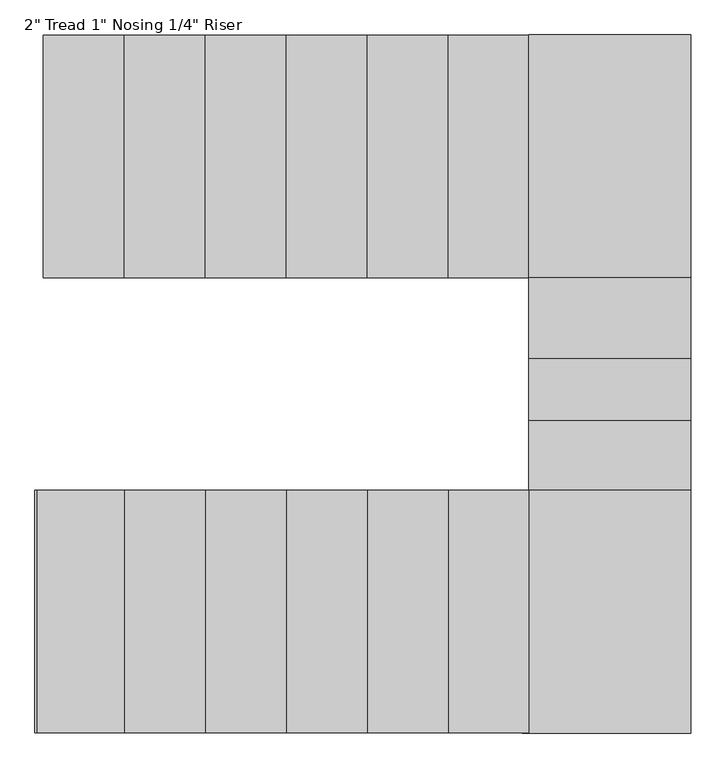
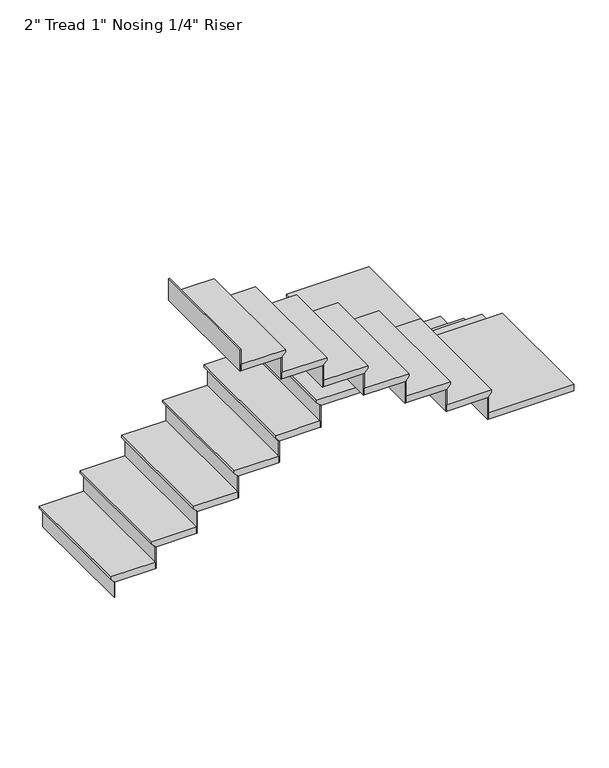
"""IFC4 building model written with IfcOpenShell, lengths in millimetres: stair flight geometry."""

from ifc_helpers import new_model, si_unit, origin, place, context, project, spatial, faceted_brep, source, transform, mapped, element, save


def stair_flight_91d3489d(model_context):
    return source(origin(), model_context, "Body", "Brep", [
        faceted_brep([(6477.0, 10054.8323212, 3198.2833333), (6477.0, 10054.8323212, 3217.3333333), (6477.0, 10969.2323212, 3217.3333333), (6477.0, 10969.2323212, 3198.2833333), (6502.4, 10054.8323212, 3172.8833333), (6502.4, 10969.2323212, 3172.8833333), (6807.2, 10054.8323212, 3217.3333333), (6807.2, 10969.2323212, 3217.3333333), (6502.4, 10969.2323212, 3166.5333333), (6807.2, 10969.2323212, 3166.5333333), (6807.2, 10054.8323212, 3166.5333333), (6502.4, 10054.8323212, 3166.5333333)], [[[0, 1, 2, 3]], [[4, 0, 3, 5]], [[2, 1, 6, 7]], [[8, 9, 10, 11]], [[2, 7, 9, 8, 5, 3]], [[8, 11, 4, 5]], [[6, 1, 0, 4, 11, 10]], [[7, 6, 10, 9]]]),
        faceted_brep([(6502.4, 10054.8323212, 3166.5333333), (6502.4, 10054.8323212, 3048.0), (6508.75, 10054.8323212, 3048.0), (6508.75, 10054.8323212, 3166.5333333), (6502.4, 10969.2323212, 3166.5333333), (6508.75, 10969.2323212, 3166.5333333), (6508.75, 10969.2323212, 3048.0), (6502.4, 10969.2323212, 3048.0)], [[[0, 1, 2, 3]], [[4, 5, 6, 7]], [[1, 0, 4, 7]], [[2, 1, 7, 6]], [[3, 2, 6, 5]], [[0, 3, 5, 4]]]),
        faceted_brep([(6807.2, 10054.8323212, 3335.8666667), (6807.2, 10054.8323212, 3166.5333333), (6813.55, 10054.8323212, 3166.5333333), (6813.55, 10054.8323212, 3335.8666667), (6807.2, 10969.2323212, 3335.8666667), (6813.55, 10969.2323212, 3335.8666667), (6813.55, 10969.2323212, 3166.5333333), (6807.2, 10969.2323212, 3166.5333333)], [[[0, 1, 2, 3]], [[4, 5, 6, 7]], [[1, 0, 4, 7]], [[2, 1, 7, 6]], [[3, 2, 6, 5]], [[0, 3, 5, 4]]]),
        faceted_brep([(6781.8, 10969.2323212, 3386.6666667), (6781.8, 10054.8323212, 3386.6666667), (7112.0, 10054.8323212, 3386.6666667), (7112.0, 10969.2323212, 3386.6666667), (6807.2, 10969.2323212, 3335.8666667), (7112.0, 10969.2323212, 3335.8666667), (7112.0, 10054.8323212, 3335.8666667), (6807.2, 10054.8323212, 3335.8666667), (6807.2, 10969.2323212, 3342.2166667), (6781.8, 10969.2323212, 3367.6166667), (6807.2, 10054.8323212, 3342.2166667), (6781.8, 10054.8323212, 3367.6166667)], [[[0, 1, 2, 3]], [[4, 5, 6, 7]], [[0, 3, 5, 4, 8, 9]], [[4, 7, 10, 8]], [[2, 1, 11, 10, 7, 6]], [[3, 2, 6, 5]], [[11, 1, 0, 9]], [[10, 11, 9, 8]]]),
        faceted_brep([(7112.0, 10054.8323212, 3505.2), (7112.0, 10054.8323212, 3335.8666667), (7118.35, 10054.8323212, 3335.8666667), (7118.35, 10054.8323212, 3505.2), (7112.0, 10969.2323212, 3505.2), (7118.35, 10969.2323212, 3505.2), (7118.35, 10969.2323212, 3335.8666667), (7112.0, 10969.2323212, 3335.8666667)], [[[0, 1, 2, 3]], [[4, 5, 6, 7]], [[1, 0, 4, 7]], [[2, 1, 7, 6]], [[3, 2, 6, 5]], [[0, 3, 5, 4]]]),
        faceted_brep([(7086.6, 10969.2323212, 3556.0), (7086.6, 10054.8323212, 3556.0), (7416.8, 10054.8323212, 3556.0), (7416.8, 10969.2323212, 3556.0), (7112.0, 10969.2323212, 3505.2), (7416.8, 10969.2323212, 3505.2), (7416.8, 10054.8323212, 3505.2), (7112.0, 10054.8323212, 3505.2), (7112.0, 10969.2323212, 3511.55), (7086.6, 10969.2323212, 3536.95), (7112.0, 10054.8323212, 3511.55), (7086.6, 10054.8323212, 3536.95)], [[[0, 1, 2, 3]], [[4, 5, 6, 7]], [[0, 3, 5, 4, 8, 9]], [[4, 7, 10, 8]], [[2, 1, 11, 10, 7, 6]], [[3, 2, 6, 5]], [[11, 1, 0, 9]], [[10, 11, 9, 8]]]),
        faceted_brep([(7416.8, 10054.8323212, 3674.5333333), (7416.8, 10054.8323212, 3505.2), (7423.15, 10054.8323212, 3505.2), (7423.15, 10054.8323212, 3674.5333333), (7416.8, 10969.2323212, 3674.5333333), (7423.15, 10969.2323212, 3674.5333333), (7423.15, 10969.2323212, 3505.2), (7416.8, 10969.2323212, 3505.2)], [[[0, 1, 2, 3]], [[4, 5, 6, 7]], [[1, 0, 4, 7]], [[2, 1, 7, 6]], [[3, 2, 6, 5]], [[0, 3, 5, 4]]]),
        faceted_brep([(7391.4, 10969.2323212, 3725.3333333), (7391.4, 10054.8323212, 3725.3333333), (7721.6, 10054.8323212, 3725.3333333), (7721.6, 10969.2323212, 3725.3333333), (7416.8, 10969.2323212, 3674.5333333), (7721.6, 10969.2323212, 3674.5333333), (7721.6, 10054.8323212, 3674.5333333), (7416.8, 10054.8323212, 3674.5333333), (7416.8, 10969.2323212, 3680.8833333), (7391.4, 10969.2323212, 3706.2833333), (7416.8, 10054.8323212, 3680.8833333), (7391.4, 10054.8323212, 3706.2833333)], [[[0, 1, 2, 3]], [[4, 5, 6, 7]], [[0, 3, 5, 4, 8, 9]], [[4, 7, 10, 8]], [[2, 1, 11, 10, 7, 6]], [[3, 2, 6, 5]], [[11, 1, 0, 9]], [[10, 11, 9, 8]]]),
        faceted_brep([(7721.6, 10054.8323212, 3843.8666667), (7721.6, 10054.8323212, 3674.5333333), (7727.95, 10054.8323212, 3674.5333333), (7727.95, 10054.8323212, 3843.8666667), (7721.6, 10969.2323212, 3843.8666667), (7727.95, 10969.2323212, 3843.8666667), (7727.95, 10969.2323212, 3674.5333333), (7721.6, 10969.2323212, 3674.5333333)], [[[0, 1, 2, 3]], [[4, 5, 6, 7]], [[1, 0, 4, 7]], [[2, 1, 7, 6]], [[3, 2, 6, 5]], [[0, 3, 5, 4]]]),
        faceted_brep([(7696.2, 10969.2323212, 3894.6666667), (7696.2, 10054.8323212, 3894.6666667), (8026.4, 10054.8323212, 3894.6666667), (8026.4, 10969.2323212, 3894.6666667), (7721.6, 10969.2323212, 3843.8666667), (8026.4, 10969.2323212, 3843.8666667), (8026.4, 10054.8323212, 3843.8666667), (7721.6, 10054.8323212, 3843.8666667), (7721.6, 10969.2323212, 3850.2166667), (7696.2, 10969.2323212, 3875.6166667), (7721.6, 10054.8323212, 3850.2166667), (7696.2, 10054.8323212, 3875.6166667)], [[[0, 1, 2, 3]], [[4, 5, 6, 7]], [[0, 3, 5, 4, 8, 9]], [[4, 7, 10, 8]], [[2, 1, 11, 10, 7, 6]], [[3, 2, 6, 5]], [[11, 1, 0, 9]], [[10, 11, 9, 8]]]),
        faceted_brep([(8026.4, 10054.8323212, 4013.2), (8026.4, 10054.8323212, 3843.8666667), (8032.75, 10054.8323212, 3843.8666667), (8032.75, 10054.8323212, 4013.2), (8026.4, 10969.2323212, 4013.2), (8032.75, 10969.2323212, 4013.2), (8032.75, 10969.2323212, 3843.8666667), (8026.4, 10969.2323212, 3843.8666667)], [[[0, 1, 2, 3]], [[4, 5, 6, 7]], [[1, 0, 4, 7]], [[2, 1, 7, 6]], [[3, 2, 6, 5]], [[0, 3, 5, 4]]]),
        faceted_brep([(8001.0, 10969.2323212, 4064.0), (8001.0, 10054.8323212, 4064.0), (8331.2, 10054.8323212, 4064.0), (8331.2, 10969.2323212, 4064.0), (8026.4, 10969.2323212, 4013.2), (8331.2, 10969.2323212, 4013.2), (8331.2, 10054.8323212, 4013.2), (8026.4, 10054.8323212, 4013.2), (8026.4, 10969.2323212, 4019.55), (8001.0, 10969.2323212, 4044.95), (8026.4, 10054.8323212, 4019.55), (8001.0, 10054.8323212, 4044.95)], [[[0, 1, 2, 3]], [[4, 5, 6, 7]], [[0, 3, 5, 4, 8, 9]], [[4, 7, 10, 8]], [[2, 1, 11, 10, 7, 6]], [[3, 2, 6, 5]], [[11, 1, 0, 9]], [[10, 11, 9, 8]]]),
        faceted_brep([(8331.2, 10054.8323212, 4182.5333333), (8331.2, 10054.8323212, 4013.2), (8337.55, 10054.8323212, 4013.2), (8337.55, 10054.8323212, 4182.5333333), (8331.2, 10969.2323212, 4182.5333333), (8337.55, 10969.2323212, 4182.5333333), (8337.55, 10969.2323212, 4013.2), (8331.2, 10969.2323212, 4013.2)], [[[0, 1, 2, 3]], [[4, 5, 6, 7]], [[1, 0, 4, 7]], [[2, 1, 7, 6]], [[3, 2, 6, 5]], [[0, 3, 5, 4]]]),
        faceted_brep([(8915.4, 10029.4323212, 4233.3333333), (8915.4, 10969.2323212, 4233.3333333), (8305.8, 10969.2323212, 4233.3333333), (8305.8, 10029.4323212, 4233.3333333), (8915.4, 10969.2323212, 4182.5333333), (8915.4, 10029.4323212, 4182.5333333), (8305.8, 10029.4323212, 4182.5333333), (8305.8, 10054.8323212, 4182.5333333), (8331.2, 10054.8323212, 4182.5333333), (8331.2, 10969.2323212, 4182.5333333), (8331.2, 10969.2323212, 4188.8833333), (8305.8, 10969.2323212, 4214.2833333), (8331.2, 10054.8323212, 4188.8833333), (8305.8, 10054.8323212, 4214.2833333)], [[[0, 1, 2, 3]], [[4, 5, 6, 7, 8, 9]], [[1, 0, 5, 4]], [[2, 1, 4, 9, 10, 11]], [[9, 8, 12, 10]], [[8, 7, 13, 12]], [[3, 2, 11, 13, 7, 6]], [[0, 3, 6, 5]], [[11, 10, 12, 13]]]),
        faceted_brep([(8305.8, 10029.4323212, 4351.8666667), (8305.8, 10029.4323212, 4182.5333333), (8305.8, 10023.0823212, 4182.5333333), (8305.8, 10023.0823212, 4351.8666667), (8915.4, 10029.4323212, 4351.8666667), (8915.4, 10023.0823212, 4351.8666667), (8915.4, 10023.0823212, 4182.5333333), (8915.4, 10029.4323212, 4182.5333333)], [[[0, 1, 2, 3]], [[4, 5, 6, 7]], [[1, 0, 4, 7]], [[2, 1, 7, 6]], [[3, 2, 6, 5]], [[0, 3, 5, 4]]]),
        faceted_brep([(8915.4, 10054.8323212, 4402.6666667), (8305.8, 10054.8323212, 4402.6666667), (8305.8, 9724.6323212, 4402.6666667), (8915.4, 9724.6323212, 4402.6666667), (8915.4, 10029.4323212, 4351.8666667), (8915.4, 9724.6323212, 4351.8666667), (8305.8, 9724.6323212, 4351.8666667), (8305.8, 10029.4323212, 4351.8666667), (8915.4, 10029.4323212, 4358.2166667), (8915.4, 10054.8323212, 4383.6166667), (8305.8, 10029.4323212, 4358.2166667), (8305.8, 10054.8323212, 4383.6166667)], [[[0, 1, 2, 3]], [[4, 5, 6, 7]], [[0, 3, 5, 4, 8, 9]], [[4, 7, 10, 8]], [[2, 1, 11, 10, 7, 6]], [[3, 2, 6, 5]], [[11, 1, 0, 9]], [[10, 11, 9, 8]]]),
        faceted_brep([(8305.8, 9724.6323212, 4521.2), (8305.8, 9724.6323212, 4351.8666667), (8305.8, 9718.2823212, 4351.8666667), (8305.8, 9718.2823212, 4521.2), (8915.4, 9724.6323212, 4521.2), (8915.4, 9718.2823212, 4521.2), (8915.4, 9718.2823212, 4351.8666667), (8915.4, 9724.6323212, 4351.8666667)], [[[0, 1, 2, 3]], [[4, 5, 6, 7]], [[1, 0, 4, 7]], [[2, 1, 7, 6]], [[3, 2, 6, 5]], [[0, 3, 5, 4]]]),
        faceted_brep([(8915.4, 9750.0323212, 4572.0), (8305.8, 9750.0323212, 4572.0), (8305.8, 9491.8832929, 4572.0), (8915.4, 9491.8832929, 4572.0), (8915.4, 9724.6323212, 4521.2), (8915.4, 9491.8832929, 4521.2), (8305.8, 9491.8832929, 4521.2), (8305.8, 9724.6323212, 4521.2), (8915.4, 9724.6323212, 4527.55), (8915.4, 9750.0323212, 4552.95), (8305.8, 9724.6323212, 4527.55), (8305.8, 9750.0323212, 4552.95)], [[[0, 1, 2, 3]], [[4, 5, 6, 7]], [[0, 3, 5, 4, 8, 9]], [[4, 7, 10, 8]], [[2, 1, 11, 10, 7, 6]], [[3, 2, 6, 5]], [[11, 1, 0, 9]], [[10, 11, 9, 8]]]),
        faceted_brep([(8305.8, 9491.8832929, 4690.5333333), (8305.8, 9491.8832929, 4521.2), (8305.8, 9485.5332929, 4521.2), (8305.8, 9485.5332929, 4690.5333333), (8915.4, 9491.8832929, 4690.5333333), (8915.4, 9485.5332929, 4690.5333333), (8915.4, 9485.5332929, 4521.2), (8915.4, 9491.8832929, 4521.2)], [[[0, 1, 2, 3]], [[4, 5, 6, 7]], [[1, 0, 4, 7]], [[2, 1, 7, 6]], [[3, 2, 6, 5]], [[0, 3, 5, 4]]]),
        faceted_brep([(8915.4, 9517.2832929, 4741.3333333), (8305.8, 9517.2832929, 4741.3333333), (8305.8, 9229.3323212, 4741.3333333), (8915.4, 9229.3323212, 4741.3333333), (8915.4, 9491.8832929, 4690.5333333), (8915.4, 9229.3323212, 4690.5333333), (8305.8, 9229.3323212, 4690.5333333), (8305.8, 9491.8832929, 4690.5333333), (8915.4, 9491.8832929, 4696.8833333), (8915.4, 9517.2832929, 4722.2833333), (8305.8, 9491.8832929, 4696.8833333), (8305.8, 9517.2832929, 4722.2833333)], [[[0, 1, 2, 3]], [[4, 5, 6, 7]], [[0, 3, 5, 4, 8, 9]], [[4, 7, 10, 8]], [[2, 1, 11, 10, 7, 6]], [[3, 2, 6, 5]], [[11, 1, 0, 9]], [[10, 11, 9, 8]]]),
        faceted_brep([(8305.8, 9229.3323212, 4859.8666667), (8305.8, 9229.3323212, 4690.5333333), (8305.8, 9222.9823212, 4690.5333333), (8305.8, 9222.9823212, 4859.8666667), (8915.4, 9229.3323212, 4859.8666667), (8915.4, 9222.9823212, 4859.8666667), (8915.4, 9222.9823212, 4690.5333333), (8915.4, 9229.3323212, 4690.5333333)], [[[0, 1, 2, 3]], [[4, 5, 6, 7]], [[1, 0, 4, 7]], [[2, 1, 7, 6]], [[3, 2, 6, 5]], [[0, 3, 5, 4]]]),
        faceted_brep([(8280.4, 8340.3323212, 4910.6666667), (8915.4, 8340.3323212, 4910.6666667), (8915.4, 9254.7323212, 4910.6666667), (8280.4, 9254.7323212, 4910.6666667), (8915.4, 8340.3323212, 4859.8666667), (8280.4, 8340.3323212, 4859.8666667), (8280.4, 9254.7323212, 4859.8666667), (8305.8, 9254.7323212, 4859.8666667), (8305.8, 9229.3323212, 4859.8666667), (8915.4, 9229.3323212, 4859.8666667), (8915.4, 9229.3323212, 4866.2166667), (8915.4, 9254.7323212, 4891.6166667), (8305.8, 9229.3323212, 4866.2166667), (8305.8, 9254.7323212, 4891.6166667)], [[[0, 1, 2, 3]], [[4, 5, 6, 7, 8, 9]], [[1, 0, 5, 4]], [[2, 1, 4, 9, 10, 11]], [[9, 8, 12, 10]], [[8, 7, 13, 12]], [[3, 2, 11, 13, 7, 6]], [[0, 3, 6, 5]], [[11, 10, 12, 13]]]),
        faceted_brep([(8280.4, 9254.7323212, 5029.2), (8280.4, 9254.7323212, 4859.8666667), (8274.05, 9254.7323212, 4859.8666667), (8274.05, 9254.7323212, 5029.2), (8280.4, 8340.3323212, 5029.2), (8274.05, 8340.3323212, 5029.2), (8274.05, 8340.3323212, 4859.8666667), (8280.4, 8340.3323212, 4859.8666667)], [[[0, 1, 2, 3]], [[4, 5, 6, 7]], [[1, 0, 4, 7]], [[2, 1, 7, 6]], [[3, 2, 6, 5]], [[0, 3, 5, 4]]]),
        faceted_brep([(8305.8, 8340.3323212, 5080.0), (8305.8, 9254.7323212, 5080.0), (7975.6, 9254.7323212, 5080.0), (7975.6, 8340.3323212, 5080.0), (8280.4, 8340.3323212, 5029.2), (7975.6, 8340.3323212, 5029.2), (7975.6, 9254.7323212, 5029.2), (8280.4, 9254.7323212, 5029.2), (8280.4, 8340.3323212, 5035.55), (8305.8, 8340.3323212, 5060.95), (8280.4, 9254.7323212, 5035.55), (8305.8, 9254.7323212, 5060.95)], [[[0, 1, 2, 3]], [[4, 5, 6, 7]], [[0, 3, 5, 4, 8, 9]], [[4, 7, 10, 8]], [[2, 1, 11, 10, 7, 6]], [[3, 2, 6, 5]], [[11, 1, 0, 9]], [[10, 11, 9, 8]]]),
        faceted_brep([(7975.6, 9254.7323212, 5198.5333333), (7975.6, 9254.7323212, 5029.2), (7969.25, 9254.7323212, 5029.2), (7969.25, 9254.7323212, 5198.5333333), (7975.6, 8340.3323212, 5198.5333333), (7969.25, 8340.3323212, 5198.5333333), (7969.25, 8340.3323212, 5029.2), (7975.6, 8340.3323212, 5029.2)], [[[0, 1, 2, 3]], [[4, 5, 6, 7]], [[1, 0, 4, 7]], [[2, 1, 7, 6]], [[3, 2, 6, 5]], [[0, 3, 5, 4]]]),
        faceted_brep([(8001.0, 8340.3323212, 5249.3333333), (8001.0, 9254.7323212, 5249.3333333), (7670.8, 9254.7323212, 5249.3333333), (7670.8, 8340.3323212, 5249.3333333), (7975.6, 8340.3323212, 5198.5333333), (7670.8, 8340.3323212, 5198.5333333), (7670.8, 9254.7323212, 5198.5333333), (7975.6, 9254.7323212, 5198.5333333), (7975.6, 8340.3323212, 5204.8833333), (8001.0, 8340.3323212, 5230.2833333), (7975.6, 9254.7323212, 5204.8833333), (8001.0, 9254.7323212, 5230.2833333)], [[[0, 1, 2, 3]], [[4, 5, 6, 7]], [[0, 3, 5, 4, 8, 9]], [[4, 7, 10, 8]], [[2, 1, 11, 10, 7, 6]], [[3, 2, 6, 5]], [[11, 1, 0, 9]], [[10, 11, 9, 8]]]),
        faceted_brep([(7670.8, 9254.7323212, 5367.8666667), (7670.8, 9254.7323212, 5198.5333333), (7664.45, 9254.7323212, 5198.5333333), (7664.45, 9254.7323212, 5367.8666667), (7670.8, 8340.3323212, 5367.8666667), (7664.45, 8340.3323212, 5367.8666667), (7664.45, 8340.3323212, 5198.5333333), (7670.8, 8340.3323212, 5198.5333333)], [[[0, 1, 2, 3]], [[4, 5, 6, 7]], [[1, 0, 4, 7]], [[2, 1, 7, 6]], [[3, 2, 6, 5]], [[0, 3, 5, 4]]]),
        faceted_brep([(7696.2, 8340.3323212, 5418.6666667), (7696.2, 9254.7323212, 5418.6666667), (7366.0, 9254.7323212, 5418.6666667), (7366.0, 8340.3323212, 5418.6666667), (7670.8, 8340.3323212, 5367.8666667), (7366.0, 8340.3323212, 5367.8666667), (7366.0, 9254.7323212, 5367.8666667), (7670.8, 9254.7323212, 5367.8666667), (7670.8, 8340.3323212, 5374.2166667), (7696.2, 8340.3323212, 5399.6166667), (7670.8, 9254.7323212, 5374.2166667), (7696.2, 9254.7323212, 5399.6166667)], [[[0, 1, 2, 3]], [[4, 5, 6, 7]], [[0, 3, 5, 4, 8, 9]], [[4, 7, 10, 8]], [[2, 1, 11, 10, 7, 6]], [[3, 2, 6, 5]], [[11, 1, 0, 9]], [[10, 11, 9, 8]]]),
        faceted_brep([(7366.0, 9254.7323212, 5537.2), (7366.0, 9254.7323212, 5367.8666667), (7359.65, 9254.7323212, 5367.8666667), (7359.65, 9254.7323212, 5537.2), (7366.0, 8340.3323212, 5537.2), (7359.65, 8340.3323212, 5537.2), (7359.65, 8340.3323212, 5367.8666667), (7366.0, 8340.3323212, 5367.8666667)], [[[0, 1, 2, 3]], [[4, 5, 6, 7]], [[1, 0, 4, 7]], [[2, 1, 7, 6]], [[3, 2, 6, 5]], [[0, 3, 5, 4]]]),
        faceted_brep([(7391.4, 8340.3323212, 5588.0), (7391.4, 9254.7323212, 5588.0), (7061.2, 9254.7323212, 5588.0), (7061.2, 8340.3323212, 5588.0), (7366.0, 8340.3323212, 5537.2), (7061.2, 8340.3323212, 5537.2), (7061.2, 9254.7323212, 5537.2), (7366.0, 9254.7323212, 5537.2), (7366.0, 8340.3323212, 5543.55), (7391.4, 8340.3323212, 5568.95), (7366.0, 9254.7323212, 5543.55), (7391.4, 9254.7323212, 5568.95)], [[[0, 1, 2, 3]], [[4, 5, 6, 7]], [[0, 3, 5, 4, 8, 9]], [[4, 7, 10, 8]], [[2, 1, 11, 10, 7, 6]], [[3, 2, 6, 5]], [[11, 1, 0, 9]], [[10, 11, 9, 8]]]),
        faceted_brep([(7061.2, 9254.7323212, 5706.5333333), (7061.2, 9254.7323212, 5537.2), (7054.85, 9254.7323212, 5537.2), (7054.85, 9254.7323212, 5706.5333333), (7061.2, 8340.3323212, 5706.5333333), (7054.85, 8340.3323212, 5706.5333333), (7054.85, 8340.3323212, 5537.2), (7061.2, 8340.3323212, 5537.2)], [[[0, 1, 2, 3]], [[4, 5, 6, 7]], [[1, 0, 4, 7]], [[2, 1, 7, 6]], [[3, 2, 6, 5]], [[0, 3, 5, 4]]]),
        faceted_brep([(7086.6, 8340.3323212, 5757.3333333), (7086.6, 9254.7323212, 5757.3333333), (6756.4, 9254.7323212, 5757.3333333), (6756.4, 8340.3323212, 5757.3333333), (7061.2, 8340.3323212, 5706.5333333), (6756.4, 8340.3323212, 5706.5333333), (6756.4, 9254.7323212, 5706.5333333), (7061.2, 9254.7323212, 5706.5333333), (7061.2, 8340.3323212, 5712.8833333), (7086.6, 8340.3323212, 5738.2833333), (7061.2, 9254.7323212, 5712.8833333), (7086.6, 9254.7323212, 5738.2833333)], [[[0, 1, 2, 3]], [[4, 5, 6, 7]], [[0, 3, 5, 4, 8, 9]], [[4, 7, 10, 8]], [[2, 1, 11, 10, 7, 6]], [[3, 2, 6, 5]], [[11, 1, 0, 9]], [[10, 11, 9, 8]]]),
        faceted_brep([(6756.4, 9254.7323212, 5875.8666667), (6756.4, 9254.7323212, 5706.5333333), (6750.05, 9254.7323212, 5706.5333333), (6750.05, 9254.7323212, 5875.8666667), (6756.4, 8340.3323212, 5875.8666667), (6750.05, 8340.3323212, 5875.8666667), (6750.05, 8340.3323212, 5706.5333333), (6756.4, 8340.3323212, 5706.5333333)], [[[0, 1, 2, 3]], [[4, 5, 6, 7]], [[1, 0, 4, 7]], [[2, 1, 7, 6]], [[3, 2, 6, 5]], [[0, 3, 5, 4]]]),
        faceted_brep([(6451.6, 9254.7323212, 6045.2), (6451.6, 9254.7323212, 5875.8666667), (6445.25, 9254.7323212, 5875.8666667), (6445.25, 9254.7323212, 6045.2), (6451.6, 8340.3323212, 6045.2), (6445.25, 8340.3323212, 6045.2), (6445.25, 8340.3323212, 5875.8666667), (6451.6, 8340.3323212, 5875.8666667)], [[[0, 1, 2, 3]], [[4, 5, 6, 7]], [[1, 0, 4, 7]], [[2, 1, 7, 6]], [[3, 2, 6, 5]], [[0, 3, 5, 4]]]),
        faceted_brep([(6781.8, 8340.3323212, 5926.6666667), (6781.8, 9254.7323212, 5926.6666667), (6451.6, 9254.7323212, 5926.6666667), (6451.6, 8340.3323212, 5926.6666667), (6756.4, 8340.3323212, 5875.8666667), (6451.6, 8340.3323212, 5875.8666667), (6451.6, 9254.7323212, 5875.8666667), (6756.4, 9254.7323212, 5875.8666667), (6756.4, 8340.3323212, 5882.2166667), (6781.8, 8340.3323212, 5907.6166667), (6756.4, 9254.7323212, 5882.2166667), (6781.8, 9254.7323212, 5907.6166667)], [[[0, 1, 2, 3]], [[4, 5, 6, 7]], [[0, 3, 5, 4, 8, 9]], [[4, 7, 10, 8]], [[2, 1, 11, 10, 7, 6]], [[3, 2, 6, 5]], [[11, 1, 0, 9]], [[10, 11, 9, 8]]]),
    ])


if __name__ == "__main__":
    model = new_model("IFC4")
    model_context = context("Model", 3, world=origin())
    ifc_project = project(units=[si_unit("LENGTHUNIT", "METRE", prefix="MILLI")], contexts=[model_context])
    site = spatial("IfcSite", under=ifc_project)
    building = spatial("IfcBuilding", under=site)
    placement = place(None, origin())
    stair_flight_shape = stair_flight_91d3489d(model_context)
    element("IfcStairFlight", 1, ObjectType="2\" Tread 1\" Nosing 1/4\" Riser", at=placement, inside=building, context=model_context, shape_type="MappedRepresentation", body=[
        mapped(stair_flight_shape, transform((0.0, 0.0, 0.0), x_axis=(1.0, 0.0, 0.0), y_axis=(0.0, 1.0, 0.0), z_axis=(0.0, 0.0, 1.0))),
    ])
    save(model, "model.ifc")
